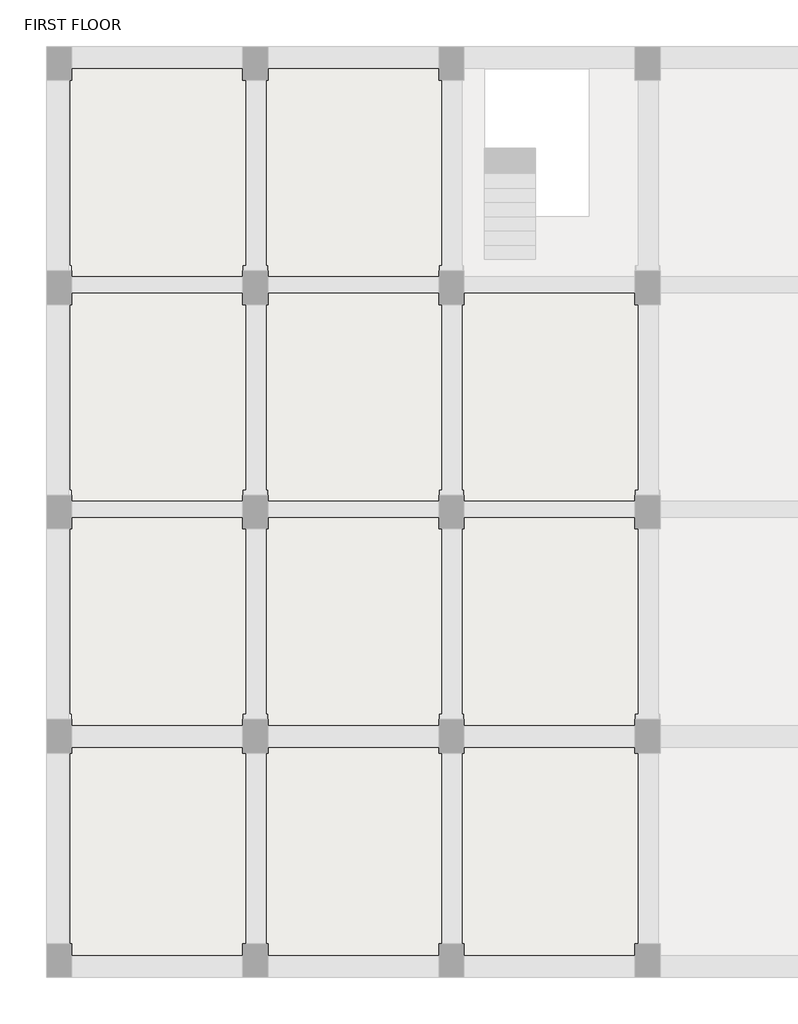
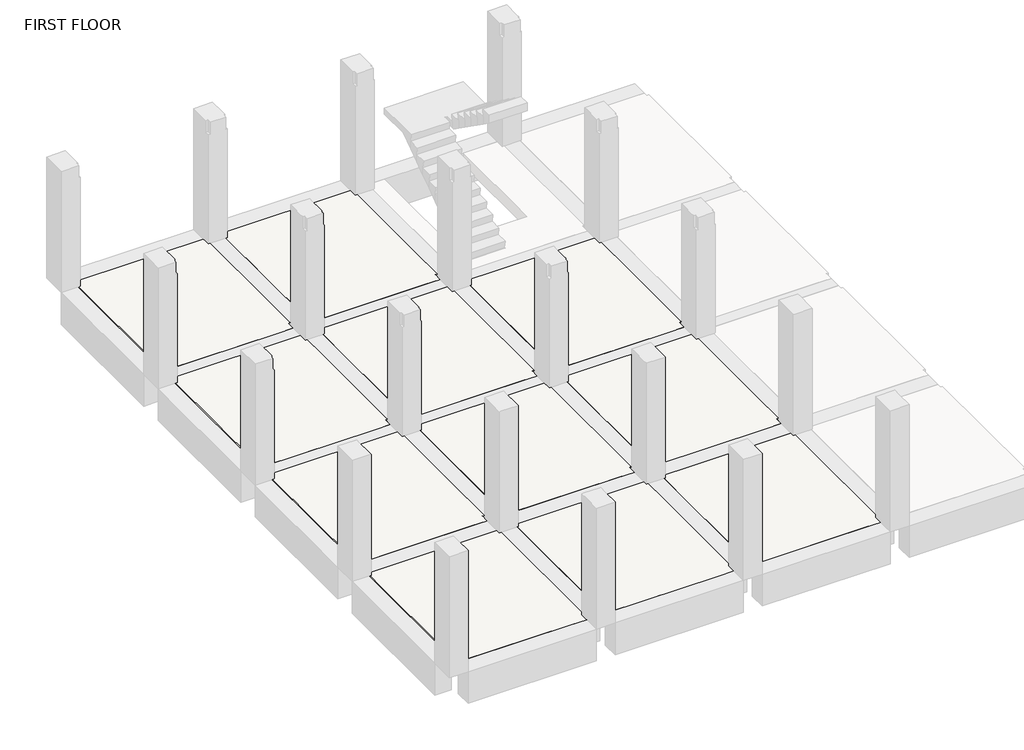
# One storey, part 1 of 4: 21 slabs.
"""IFC4 building model written with IfcOpenShell, lengths in millimetres."""

from ifc_helpers import new_model, si_unit, origin, place, context, project, spatial, faceted_brep, element, save

model = new_model("IFC4")

# Units and contexts
model_context = context("Model", 3, world=origin())
ifc_project = project(units=[si_unit("LENGTHUNIT", "METRE", prefix="MILLI")], contexts=[model_context])

# Site, building, storey
site = spatial("IfcSite", under=ifc_project)
building = spatial("IfcBuilding", under=site)
storey = spatial("IfcBuildingStorey", under=building, Name="FIRST FLOOR", Elevation=3048.0)

# Slabs
placement = place(None, origin())
element("IfcSlab", 1, ObjectType="Generic 300mm", at=placement, inside=storey, context=model_context, shape_type="Brep", body=[
    faceted_brep([(955.1115906, 11203.1212443, 2748.0), (955.1115906, 11103.1212443, 2748.0), (955.1115906, 7803.1212443, 2748.0), (930.1115906, 7803.1212443, 2748.0), (905.1115906, 7803.1212443, 2748.0), (905.1115906, 7603.1212443, 2748.0), (530.1115906, 7603.1212443, 2748.0), (-2144.8884094, 7603.1212443, 2748.0), (-2144.8884094, 7803.1212443, 2748.0), (-2169.8884094, 7803.1212443, 2748.0), (-2169.8884094, 11103.1212443, 2748.0), (-2169.8884094, 11203.1212443, 2748.0), (-2144.8884094, 11203.1212443, 2748.0), (-2144.8884094, 11303.1212443, 2748.0), (905.1115906, 11303.1212443, 2748.0), (905.1115906, 11203.1212443, 2748.0), (955.1115906, 11203.1212443, 3048.0), (905.1115906, 11203.1212443, 3048.0), (905.1115906, 11303.1212443, 3048.0), (-2144.8884094, 11303.1212443, 3048.0), (-2144.8884094, 11203.1212443, 3048.0), (-2169.8884094, 11203.1212443, 3048.0), (-2169.8884094, 11103.1212443, 3048.0), (-2169.8884094, 7803.1212443, 3048.0), (-2144.8884094, 7803.1212443, 3048.0), (-2144.8884094, 7703.1212443, 3048.0), (-2144.8884094, 7603.1212443, 3048.0), (530.1115906, 7603.1212443, 3048.0), (905.1115906, 7603.1212443, 3048.0), (905.1115906, 7703.1212443, 3048.0), (905.1115906, 7803.1212443, 3048.0), (930.1115906, 7803.1212443, 3048.0), (955.1115906, 7803.1212443, 3048.0), (955.1115906, 11103.1212443, 3048.0)], [[[0, 1, 2, 3, 4, 5, 6, 7, 8, 9, 10, 11, 12, 13, 14, 15]], [[16, 17, 18, 19, 20, 21, 22, 23, 24, 25, 26, 27, 28, 29, 30, 31, 32, 33]], [[2, 1, 0, 16, 33, 32]], [[4, 3, 2, 32, 31, 30]], [[5, 4, 30, 29, 28]], [[6, 5, 28, 27]], [[7, 6, 27, 26]], [[8, 7, 26, 25, 24]], [[9, 8, 24, 23]], [[11, 10, 9, 23, 22, 21]], [[12, 11, 21, 20]], [[13, 12, 20, 19]], [[14, 13, 19, 18]], [[15, 14, 18, 17]], [[0, 15, 17, 16]]]),
])
element("IfcSlab", 2, ObjectType="Generic 300mm", at=placement, inside=storey, context=model_context, shape_type="Brep", body=[
    faceted_brep([(-2544.8884094, 11203.1212443, 2748.0), (-2544.8884094, 11103.1212443, 2748.0), (-2544.8884094, 7803.1212443, 2748.0), (-2569.8884094, 7803.1212443, 2748.0), (-2594.8884094, 7803.1212443, 2748.0), (-2594.8884094, 7603.1212443, 2748.0), (-2969.8884094, 7603.1212443, 2748.0), (-5644.8884094, 7603.1212443, 2748.0), (-5644.8884094, 7803.1212443, 2748.0), (-5669.8884094, 7803.1212443, 2748.0), (-5669.8884094, 11103.1212443, 2748.0), (-5669.8884094, 11203.1212443, 2748.0), (-5644.8884094, 11203.1212443, 2748.0), (-5644.8884094, 11303.1212443, 2748.0), (-2594.8884094, 11303.1212443, 2748.0), (-2594.8884094, 11203.1212443, 2748.0), (-2544.8884094, 11203.1212443, 3048.0), (-2594.8884094, 11203.1212443, 3048.0), (-2594.8884094, 11303.1212443, 3048.0), (-5644.8884094, 11303.1212443, 3048.0), (-5644.8884094, 11203.1212443, 3048.0), (-5669.8884094, 11203.1212443, 3048.0), (-5669.8884094, 11103.1212443, 3048.0), (-5669.8884094, 7803.1212443, 3048.0), (-5644.8884094, 7803.1212443, 3048.0), (-5644.8884094, 7703.1212443, 3048.0), (-5644.8884094, 7603.1212443, 3048.0), (-2969.8884094, 7603.1212443, 3048.0), (-2594.8884094, 7603.1212443, 3048.0), (-2594.8884094, 7703.1212443, 3048.0), (-2594.8884094, 7803.1212443, 3048.0), (-2569.8884094, 7803.1212443, 3048.0), (-2544.8884094, 7803.1212443, 3048.0), (-2544.8884094, 11103.1212443, 3048.0)], [[[0, 1, 2, 3, 4, 5, 6, 7, 8, 9, 10, 11, 12, 13, 14, 15]], [[16, 17, 18, 19, 20, 21, 22, 23, 24, 25, 26, 27, 28, 29, 30, 31, 32, 33]], [[2, 1, 0, 16, 33, 32]], [[4, 3, 2, 32, 31, 30]], [[5, 4, 30, 29, 28]], [[6, 5, 28, 27]], [[7, 6, 27, 26]], [[8, 7, 26, 25, 24]], [[9, 8, 24, 23]], [[11, 10, 9, 23, 22, 21]], [[12, 11, 21, 20]], [[13, 12, 20, 19]], [[14, 13, 19, 18]], [[15, 14, 18, 17]], [[0, 15, 17, 16]]]),
])
element("IfcSlab", 3, ObjectType="Generic 300mm", at=placement, inside=storey, context=model_context, shape_type="Brep", body=[
    faceted_brep([(-6044.8884094, 11203.1212443, 2748.0), (-6044.8884094, 11103.1212443, 2748.0), (-6044.8884094, 7803.1212443, 2748.0), (-6069.8884094, 7803.1212443, 2748.0), (-6094.8884094, 7803.1212443, 2748.0), (-6094.8884094, 7603.1212443, 2748.0), (-6469.8884094, 7603.1212443, 2748.0), (-9144.8884094, 7603.1212443, 2748.0), (-9144.8884094, 7803.1212443, 2748.0), (-9169.8884094, 7803.1212443, 2748.0), (-9169.8884094, 11103.1212443, 2748.0), (-9169.8884094, 11203.1212443, 2748.0), (-9144.8884094, 11203.1212443, 2748.0), (-9144.8884094, 11303.1212443, 2748.0), (-6094.8884094, 11303.1212443, 2748.0), (-6094.8884094, 11203.1212443, 2748.0), (-6044.8884094, 11203.1212443, 3048.0), (-6094.8884094, 11203.1212443, 3048.0), (-6094.8884094, 11303.1212443, 3048.0), (-9144.8884094, 11303.1212443, 3048.0), (-9144.8884094, 11203.1212443, 3048.0), (-9169.8884094, 11203.1212443, 3048.0), (-9169.8884094, 11103.1212443, 3048.0), (-9169.8884094, 7803.1212443, 3048.0), (-9144.8884094, 7803.1212443, 3048.0), (-9144.8884094, 7703.1212443, 3048.0), (-9144.8884094, 7603.1212443, 3048.0), (-6469.8884094, 7603.1212443, 3048.0), (-6094.8884094, 7603.1212443, 3048.0), (-6094.8884094, 7703.1212443, 3048.0), (-6094.8884094, 7803.1212443, 3048.0), (-6069.8884094, 7803.1212443, 3048.0), (-6044.8884094, 7803.1212443, 3048.0), (-6044.8884094, 11103.1212443, 3048.0)], [[[0, 1, 2, 3, 4, 5, 6, 7, 8, 9, 10, 11, 12, 13, 14, 15]], [[16, 17, 18, 19, 20, 21, 22, 23, 24, 25, 26, 27, 28, 29, 30, 31, 32, 33]], [[2, 1, 0, 16, 33, 32]], [[4, 3, 2, 32, 31, 30]], [[5, 4, 30, 29, 28]], [[6, 5, 28, 27]], [[7, 6, 27, 26]], [[8, 7, 26, 25, 24]], [[9, 8, 24, 23]], [[11, 10, 9, 23, 22, 21]], [[12, 11, 21, 20]], [[13, 12, 20, 19]], [[14, 13, 19, 18]], [[15, 14, 18, 17]], [[0, 15, 17, 16]]]),
])
element("IfcSlab", 4, ObjectType="Generic 300mm", at=placement, inside=storey, context=model_context, shape_type="Brep", body=[
    faceted_brep([(-6044.8884094, 7103.1212443, 2748.0), (-6044.8884094, 3703.1212443, 2748.0), (-6069.8884094, 3703.1212443, 2748.0), (-6094.8884094, 3703.1212443, 2748.0), (-6094.8884094, 3503.1212443, 2748.0), (-6469.8884094, 3503.1212443, 2748.0), (-9144.8884094, 3503.1212443, 2748.0), (-9144.8884094, 3703.1212443, 2748.0), (-9169.8884094, 3703.1212443, 2748.0), (-9169.8884094, 7103.1212443, 2748.0), (-9144.8884094, 7103.1212443, 2748.0), (-9144.8884094, 7203.1212443, 2748.0), (-6094.8884094, 7203.1212443, 2748.0), (-6094.8884094, 7103.1212443, 2748.0), (-6069.8884094, 7103.1212443, 2748.0), (-6044.8884094, 7103.1212443, 3048.0), (-6094.8884094, 7103.1212443, 3048.0), (-6094.8884094, 7203.1212443, 3048.0), (-9144.8884094, 7203.1212443, 3048.0), (-9144.8884094, 7103.1212443, 3048.0), (-9169.8884094, 7103.1212443, 3048.0), (-9169.8884094, 3703.1212443, 3048.0), (-9144.8884094, 3703.1212443, 3048.0), (-9144.8884094, 3503.1212443, 3048.0), (-6469.8884094, 3503.1212443, 3048.0), (-6094.8884094, 3503.1212443, 3048.0), (-6094.8884094, 3703.1212443, 3048.0), (-6044.8884094, 3703.1212443, 3048.0)], [[[0, 1, 2, 3, 4, 5, 6, 7, 8, 9, 10, 11, 12, 13, 14]], [[15, 16, 17, 18, 19, 20, 21, 22, 23, 24, 25, 26, 27]], [[1, 0, 15, 27]], [[3, 2, 1, 27, 26]], [[4, 3, 26, 25]], [[5, 4, 25, 24]], [[6, 5, 24, 23]], [[7, 6, 23, 22]], [[8, 7, 22, 21]], [[9, 8, 21, 20]], [[10, 9, 20, 19]], [[11, 10, 19, 18]], [[12, 11, 18, 17]], [[13, 12, 17, 16]], [[0, 14, 13, 16, 15]]]),
])
element("IfcSlab", 5, ObjectType="Generic 300mm", at=placement, inside=storey, context=model_context, shape_type="Brep", body=[
    faceted_brep([(-2544.8884094, 7103.1212443, 2748.0), (-2544.8884094, 3703.1212443, 2748.0), (-2569.8884094, 3703.1212443, 2748.0), (-2594.8884094, 3703.1212443, 2748.0), (-2594.8884094, 3503.1212443, 2748.0), (-2969.8884094, 3503.1212443, 2748.0), (-5644.8884094, 3503.1212443, 2748.0), (-5644.8884094, 3703.1212443, 2748.0), (-5669.8884094, 3703.1212443, 2748.0), (-5669.8884094, 7103.1212443, 2748.0), (-5644.8884094, 7103.1212443, 2748.0), (-5644.8884094, 7203.1212443, 2748.0), (-2594.8884094, 7203.1212443, 2748.0), (-2594.8884094, 7103.1212443, 2748.0), (-2569.8884094, 7103.1212443, 2748.0), (-2544.8884094, 7103.1212443, 3048.0), (-2594.8884094, 7103.1212443, 3048.0), (-2594.8884094, 7203.1212443, 3048.0), (-5644.8884094, 7203.1212443, 3048.0), (-5644.8884094, 7103.1212443, 3048.0), (-5669.8884094, 7103.1212443, 3048.0), (-5669.8884094, 3703.1212443, 3048.0), (-5644.8884094, 3703.1212443, 3048.0), (-5644.8884094, 3503.1212443, 3048.0), (-2969.8884094, 3503.1212443, 3048.0), (-2594.8884094, 3503.1212443, 3048.0), (-2594.8884094, 3703.1212443, 3048.0), (-2544.8884094, 3703.1212443, 3048.0)], [[[0, 1, 2, 3, 4, 5, 6, 7, 8, 9, 10, 11, 12, 13, 14]], [[15, 16, 17, 18, 19, 20, 21, 22, 23, 24, 25, 26, 27]], [[1, 0, 15, 27]], [[3, 2, 1, 27, 26]], [[4, 3, 26, 25]], [[5, 4, 25, 24]], [[6, 5, 24, 23]], [[7, 6, 23, 22]], [[8, 7, 22, 21]], [[9, 8, 21, 20]], [[10, 9, 20, 19]], [[11, 10, 19, 18]], [[12, 11, 18, 17]], [[13, 12, 17, 16]], [[0, 14, 13, 16, 15]]]),
])
element("IfcSlab", 6, ObjectType="Generic 300mm", at=placement, inside=storey, context=model_context, shape_type="Brep", body=[
    faceted_brep([(955.1115906, 7103.1212443, 2748.0), (955.1115906, 3703.1212443, 2748.0), (930.1115906, 3703.1212443, 2748.0), (905.1115906, 3703.1212443, 2748.0), (905.1115906, 3503.1212443, 2748.0), (530.1115906, 3503.1212443, 2748.0), (-2144.8884094, 3503.1212443, 2748.0), (-2144.8884094, 3703.1212443, 2748.0), (-2169.8884094, 3703.1212443, 2748.0), (-2169.8884094, 7103.1212443, 2748.0), (-2144.8884094, 7103.1212443, 2748.0), (-2144.8884094, 7203.1212443, 2748.0), (905.1115906, 7203.1212443, 2748.0), (905.1115906, 7103.1212443, 2748.0), (930.1115906, 7103.1212443, 2748.0), (955.1115906, 7103.1212443, 3048.0), (905.1115906, 7103.1212443, 3048.0), (905.1115906, 7203.1212443, 3048.0), (-2144.8884094, 7203.1212443, 3048.0), (-2144.8884094, 7103.1212443, 3048.0), (-2169.8884094, 7103.1212443, 3048.0), (-2169.8884094, 3703.1212443, 3048.0), (-2144.8884094, 3703.1212443, 3048.0), (-2144.8884094, 3503.1212443, 3048.0), (530.1115906, 3503.1212443, 3048.0), (905.1115906, 3503.1212443, 3048.0), (905.1115906, 3703.1212443, 3048.0), (955.1115906, 3703.1212443, 3048.0)], [[[0, 1, 2, 3, 4, 5, 6, 7, 8, 9, 10, 11, 12, 13, 14]], [[15, 16, 17, 18, 19, 20, 21, 22, 23, 24, 25, 26, 27]], [[1, 0, 15, 27]], [[3, 2, 1, 27, 26]], [[4, 3, 26, 25]], [[5, 4, 25, 24]], [[6, 5, 24, 23]], [[7, 6, 23, 22]], [[8, 7, 22, 21]], [[9, 8, 21, 20]], [[10, 9, 20, 19]], [[11, 10, 19, 18]], [[12, 11, 18, 17]], [[13, 12, 17, 16]], [[0, 14, 13, 16, 15]]]),
])
element("IfcSlab", 7, ObjectType="Generic 300mm", at=placement, inside=storey, context=model_context, shape_type="Brep", body=[
    faceted_brep([(955.1115906, 15203.1212443, 2748.0), (955.1115906, 15103.1212443, 2748.0), (955.1115906, 11803.1212443, 2748.0), (930.1115906, 11803.1212443, 2748.0), (905.1115906, 11803.1212443, 2748.0), (905.1115906, 11603.1212443, 2748.0), (530.1115906, 11603.1212443, 2748.0), (-2144.8884094, 11603.1212443, 2748.0), (-2144.8884094, 11803.1212443, 2748.0), (-2169.8884094, 11803.1212443, 2748.0), (-2169.8884094, 15103.1212443, 2748.0), (-2169.8884094, 15203.1212443, 2748.0), (-2144.8884094, 15203.1212443, 2748.0), (-2144.8884094, 15303.1212443, 2748.0), (905.1115906, 15303.1212443, 2748.0), (905.1115906, 15203.1212443, 2748.0), (955.1115906, 15203.1212443, 3048.0), (905.1115906, 15203.1212443, 3048.0), (905.1115906, 15303.1212443, 3048.0), (-2144.8884094, 15303.1212443, 3048.0), (-2144.8884094, 15203.1212443, 3048.0), (-2169.8884094, 15203.1212443, 3048.0), (-2169.8884094, 15103.1212443, 3048.0), (-2169.8884094, 11803.1212443, 3048.0), (-2144.8884094, 11803.1212443, 3048.0), (-2144.8884094, 11703.1212443, 3048.0), (-2144.8884094, 11603.1212443, 3048.0), (530.1115906, 11603.1212443, 3048.0), (905.1115906, 11603.1212443, 3048.0), (905.1115906, 11703.1212443, 3048.0), (905.1115906, 11803.1212443, 3048.0), (930.1115906, 11803.1212443, 3048.0), (955.1115906, 11803.1212443, 3048.0), (955.1115906, 15103.1212443, 3048.0)], [[[0, 1, 2, 3, 4, 5, 6, 7, 8, 9, 10, 11, 12, 13, 14, 15]], [[16, 17, 18, 19, 20, 21, 22, 23, 24, 25, 26, 27, 28, 29, 30, 31, 32, 33]], [[2, 1, 0, 16, 33, 32]], [[4, 3, 2, 32, 31, 30]], [[5, 4, 30, 29, 28]], [[6, 5, 28, 27]], [[7, 6, 27, 26]], [[8, 7, 26, 25, 24]], [[9, 8, 24, 23]], [[11, 10, 9, 23, 22, 21]], [[12, 11, 21, 20]], [[13, 12, 20, 19]], [[14, 13, 19, 18]], [[15, 14, 18, 17]], [[0, 15, 17, 16]]]),
])
element("IfcSlab", 8, ObjectType="Generic 300mm", at=placement, inside=storey, context=model_context, shape_type="Brep", body=[
    faceted_brep([(-2544.8884094, 19203.1212443, 2748.0), (-2544.8884094, 19103.1212443, 2748.0), (-2544.8884094, 15803.1212443, 2748.0), (-2569.8884094, 15803.1212443, 2748.0), (-2594.8884094, 15803.1212443, 2748.0), (-2594.8884094, 15603.1212443, 2748.0), (-2969.8884094, 15603.1212443, 2748.0), (-5644.8884094, 15603.1212443, 2748.0), (-5644.8884094, 15803.1212443, 2748.0), (-5669.8884094, 15803.1212443, 2748.0), (-5669.8884094, 19103.1212443, 2748.0), (-5669.8884094, 19203.1212443, 2748.0), (-5644.8884094, 19203.1212443, 2748.0), (-5644.8884094, 19303.1212443, 2748.0), (-2594.8884094, 19303.1212443, 2748.0), (-2594.8884094, 19203.1212443, 2748.0), (-2544.8884094, 19203.1212443, 3048.0), (-2594.8884094, 19203.1212443, 3048.0), (-2594.8884094, 19303.1212443, 3048.0), (-5644.8884094, 19303.1212443, 3048.0), (-5644.8884094, 19203.1212443, 3048.0), (-5669.8884094, 19203.1212443, 3048.0), (-5669.8884094, 19103.1212443, 3048.0), (-5669.8884094, 15803.1212443, 3048.0), (-5644.8884094, 15803.1212443, 3048.0), (-5644.8884094, 15703.1212443, 3048.0), (-5644.8884094, 15603.1212443, 3048.0), (-2969.8884094, 15603.1212443, 3048.0), (-2594.8884094, 15603.1212443, 3048.0), (-2594.8884094, 15703.1212443, 3048.0), (-2594.8884094, 15803.1212443, 3048.0), (-2569.8884094, 15803.1212443, 3048.0), (-2544.8884094, 15803.1212443, 3048.0), (-2544.8884094, 19103.1212443, 3048.0)], [[[0, 1, 2, 3, 4, 5, 6, 7, 8, 9, 10, 11, 12, 13, 14, 15]], [[16, 17, 18, 19, 20, 21, 22, 23, 24, 25, 26, 27, 28, 29, 30, 31, 32, 33]], [[2, 1, 0, 16, 33, 32]], [[4, 3, 2, 32, 31, 30]], [[5, 4, 30, 29, 28]], [[6, 5, 28, 27]], [[7, 6, 27, 26]], [[8, 7, 26, 25, 24]], [[9, 8, 24, 23]], [[11, 10, 9, 23, 22, 21]], [[12, 11, 21, 20]], [[13, 12, 20, 19]], [[14, 13, 19, 18]], [[15, 14, 18, 17]], [[0, 15, 17, 16]]]),
])
element("IfcSlab", 9, ObjectType="Generic 300mm", at=placement, inside=storey, context=model_context, shape_type="Brep", body=[
    faceted_brep([(-6044.8884094, 19203.1212443, 2748.0), (-6044.8884094, 19103.1212443, 2748.0), (-6044.8884094, 15803.1212443, 2748.0), (-6069.8884094, 15803.1212443, 2748.0), (-6094.8884094, 15803.1212443, 2748.0), (-6094.8884094, 15603.1212443, 2748.0), (-6469.8884094, 15603.1212443, 2748.0), (-9144.8884094, 15603.1212443, 2748.0), (-9144.8884094, 15803.1212443, 2748.0), (-9169.8884094, 15803.1212443, 2748.0), (-9169.8884094, 19103.1212443, 2748.0), (-9169.8884094, 19203.1212443, 2748.0), (-9144.8884094, 19203.1212443, 2748.0), (-9144.8884094, 19303.1212443, 2748.0), (-6094.8884094, 19303.1212443, 2748.0), (-6094.8884094, 19203.1212443, 2748.0), (-6044.8884094, 19203.1212443, 3048.0), (-6094.8884094, 19203.1212443, 3048.0), (-6094.8884094, 19303.1212443, 3048.0), (-9144.8884094, 19303.1212443, 3048.0), (-9144.8884094, 19203.1212443, 3048.0), (-9169.8884094, 19203.1212443, 3048.0), (-9169.8884094, 19103.1212443, 3048.0), (-9169.8884094, 15803.1212443, 3048.0), (-9144.8884094, 15803.1212443, 3048.0), (-9144.8884094, 15703.1212443, 3048.0), (-9144.8884094, 15603.1212443, 3048.0), (-6469.8884094, 15603.1212443, 3048.0), (-6094.8884094, 15603.1212443, 3048.0), (-6094.8884094, 15703.1212443, 3048.0), (-6094.8884094, 15803.1212443, 3048.0), (-6069.8884094, 15803.1212443, 3048.0), (-6044.8884094, 15803.1212443, 3048.0), (-6044.8884094, 19103.1212443, 3048.0)], [[[0, 1, 2, 3, 4, 5, 6, 7, 8, 9, 10, 11, 12, 13, 14, 15]], [[16, 17, 18, 19, 20, 21, 22, 23, 24, 25, 26, 27, 28, 29, 30, 31, 32, 33]], [[2, 1, 0, 16, 33, 32]], [[4, 3, 2, 32, 31, 30]], [[5, 4, 30, 29, 28]], [[6, 5, 28, 27]], [[7, 6, 27, 26]], [[8, 7, 26, 25, 24]], [[9, 8, 24, 23]], [[11, 10, 9, 23, 22, 21]], [[12, 11, 21, 20]], [[13, 12, 20, 19]], [[14, 13, 19, 18]], [[15, 14, 18, 17]], [[0, 15, 17, 16]]]),
])
element("IfcSlab", 10, ObjectType="Generic 300mm", at=placement, inside=storey, context=model_context, shape_type="Brep", body=[
    faceted_brep([(-6044.8884094, 15203.1212443, 2748.0), (-6044.8884094, 15103.1212443, 2748.0), (-6044.8884094, 11803.1212443, 2748.0), (-6069.8884094, 11803.1212443, 2748.0), (-6094.8884094, 11803.1212443, 2748.0), (-6094.8884094, 11603.1212443, 2748.0), (-6469.8884094, 11603.1212443, 2748.0), (-9144.8884094, 11603.1212443, 2748.0), (-9144.8884094, 11803.1212443, 2748.0), (-9169.8884094, 11803.1212443, 2748.0), (-9169.8884094, 15103.1212443, 2748.0), (-9169.8884094, 15203.1212443, 2748.0), (-9144.8884094, 15203.1212443, 2748.0), (-9144.8884094, 15303.1212443, 2748.0), (-6094.8884094, 15303.1212443, 2748.0), (-6094.8884094, 15203.1212443, 2748.0), (-6044.8884094, 15203.1212443, 3048.0), (-6094.8884094, 15203.1212443, 3048.0), (-6094.8884094, 15303.1212443, 3048.0), (-9144.8884094, 15303.1212443, 3048.0), (-9144.8884094, 15203.1212443, 3048.0), (-9169.8884094, 15203.1212443, 3048.0), (-9169.8884094, 15103.1212443, 3048.0), (-9169.8884094, 11803.1212443, 3048.0), (-9144.8884094, 11803.1212443, 3048.0), (-9144.8884094, 11703.1212443, 3048.0), (-9144.8884094, 11603.1212443, 3048.0), (-6469.8884094, 11603.1212443, 3048.0), (-6094.8884094, 11603.1212443, 3048.0), (-6094.8884094, 11703.1212443, 3048.0), (-6094.8884094, 11803.1212443, 3048.0), (-6069.8884094, 11803.1212443, 3048.0), (-6044.8884094, 11803.1212443, 3048.0), (-6044.8884094, 15103.1212443, 3048.0)], [[[0, 1, 2, 3, 4, 5, 6, 7, 8, 9, 10, 11, 12, 13, 14, 15]], [[16, 17, 18, 19, 20, 21, 22, 23, 24, 25, 26, 27, 28, 29, 30, 31, 32, 33]], [[2, 1, 0, 16, 33, 32]], [[4, 3, 2, 32, 31, 30]], [[5, 4, 30, 29, 28]], [[6, 5, 28, 27]], [[7, 6, 27, 26]], [[8, 7, 26, 25, 24]], [[9, 8, 24, 23]], [[11, 10, 9, 23, 22, 21]], [[12, 11, 21, 20]], [[13, 12, 20, 19]], [[14, 13, 19, 18]], [[15, 14, 18, 17]], [[0, 15, 17, 16]]]),
])
element("IfcSlab", 11, ObjectType="Generic 300mm", at=placement, inside=storey, context=model_context, shape_type="Brep", body=[
    faceted_brep([(-2544.8884094, 15203.1212443, 2748.0), (-2544.8884094, 15103.1212443, 2748.0), (-2544.8884094, 11803.1212443, 2748.0), (-2569.8884094, 11803.1212443, 2748.0), (-2594.8884094, 11803.1212443, 2748.0), (-2594.8884094, 11603.1212443, 2748.0), (-2969.8884094, 11603.1212443, 2748.0), (-5644.8884094, 11603.1212443, 2748.0), (-5644.8884094, 11803.1212443, 2748.0), (-5669.8884094, 11803.1212443, 2748.0), (-5669.8884094, 15103.1212443, 2748.0), (-5669.8884094, 15203.1212443, 2748.0), (-5644.8884094, 15203.1212443, 2748.0), (-5644.8884094, 15303.1212443, 2748.0), (-2594.8884094, 15303.1212443, 2748.0), (-2594.8884094, 15203.1212443, 2748.0), (-2544.8884094, 15203.1212443, 3048.0), (-2594.8884094, 15203.1212443, 3048.0), (-2594.8884094, 15303.1212443, 3048.0), (-5644.8884094, 15303.1212443, 3048.0), (-5644.8884094, 15203.1212443, 3048.0), (-5669.8884094, 15203.1212443, 3048.0), (-5669.8884094, 15103.1212443, 3048.0), (-5669.8884094, 11803.1212443, 3048.0), (-5644.8884094, 11803.1212443, 3048.0), (-5644.8884094, 11703.1212443, 3048.0), (-5644.8884094, 11603.1212443, 3048.0), (-2969.8884094, 11603.1212443, 3048.0), (-2594.8884094, 11603.1212443, 3048.0), (-2594.8884094, 11703.1212443, 3048.0), (-2594.8884094, 11803.1212443, 3048.0), (-2569.8884094, 11803.1212443, 3048.0), (-2544.8884094, 11803.1212443, 3048.0), (-2544.8884094, 15103.1212443, 3048.0)], [[[0, 1, 2, 3, 4, 5, 6, 7, 8, 9, 10, 11, 12, 13, 14, 15]], [[16, 17, 18, 19, 20, 21, 22, 23, 24, 25, 26, 27, 28, 29, 30, 31, 32, 33]], [[2, 1, 0, 16, 33, 32]], [[4, 3, 2, 32, 31, 30]], [[5, 4, 30, 29, 28]], [[6, 5, 28, 27]], [[7, 6, 27, 26]], [[8, 7, 26, 25, 24]], [[9, 8, 24, 23]], [[11, 10, 9, 23, 22, 21]], [[12, 11, 21, 20]], [[13, 12, 20, 19]], [[14, 13, 19, 18]], [[15, 14, 18, 17]], [[0, 15, 17, 16]]]),
])
element("IfcSlab", 12, ObjectType="Generic 300mm", at=placement, inside=storey, context=model_context, shape_type="Brep", body=[
    faceted_brep([(955.1115906, 11203.1212443, 2748.0), (955.1115906, 11103.1212443, 2748.0), (955.1115906, 7803.1212443, 2748.0), (930.1115906, 7803.1212443, 2748.0), (905.1115906, 7803.1212443, 2748.0), (905.1115906, 7603.1212443, 2748.0), (530.1115906, 7603.1212443, 2748.0), (-2144.8884094, 7603.1212443, 2748.0), (-2144.8884094, 7803.1212443, 2748.0), (-2169.8884094, 7803.1212443, 2748.0), (-2169.8884094, 11103.1212443, 2748.0), (-2169.8884094, 11203.1212443, 2748.0), (-2144.8884094, 11203.1212443, 2748.0), (-2144.8884094, 11303.1212443, 2748.0), (905.1115906, 11303.1212443, 2748.0), (905.1115906, 11203.1212443, 2748.0), (955.1115906, 11203.1212443, 3048.0), (905.1115906, 11203.1212443, 3048.0), (905.1115906, 11303.1212443, 3048.0), (-2144.8884094, 11303.1212443, 3048.0), (-2144.8884094, 11203.1212443, 3048.0), (-2169.8884094, 11203.1212443, 3048.0), (-2169.8884094, 11103.1212443, 3048.0), (-2169.8884094, 7803.1212443, 3048.0), (-2144.8884094, 7803.1212443, 3048.0), (-2144.8884094, 7703.1212443, 3048.0), (-2144.8884094, 7603.1212443, 3048.0), (530.1115906, 7603.1212443, 3048.0), (905.1115906, 7603.1212443, 3048.0), (905.1115906, 7703.1212443, 3048.0), (905.1115906, 7803.1212443, 3048.0), (930.1115906, 7803.1212443, 3048.0), (955.1115906, 7803.1212443, 3048.0), (955.1115906, 11103.1212443, 3048.0)], [[[0, 1, 2, 3, 4, 5, 6, 7, 8, 9, 10, 11, 12, 13, 14, 15]], [[16, 17, 18, 19, 20, 21, 22, 23, 24, 25, 26, 27, 28, 29, 30, 31, 32, 33]], [[2, 1, 0, 16, 33, 32]], [[4, 3, 2, 32, 31, 30]], [[5, 4, 30, 29, 28]], [[6, 5, 28, 27]], [[7, 6, 27, 26]], [[8, 7, 26, 25, 24]], [[9, 8, 24, 23]], [[11, 10, 9, 23, 22, 21]], [[12, 11, 21, 20]], [[13, 12, 20, 19]], [[14, 13, 19, 18]], [[15, 14, 18, 17]], [[0, 15, 17, 16]]]),
])
element("IfcSlab", 13, ObjectType="Generic 300mm", at=placement, inside=storey, context=model_context, shape_type="Brep", body=[
    faceted_brep([(-2544.8884094, 11203.1212443, 2748.0), (-2544.8884094, 11103.1212443, 2748.0), (-2544.8884094, 7803.1212443, 2748.0), (-2569.8884094, 7803.1212443, 2748.0), (-2594.8884094, 7803.1212443, 2748.0), (-2594.8884094, 7603.1212443, 2748.0), (-2969.8884094, 7603.1212443, 2748.0), (-5644.8884094, 7603.1212443, 2748.0), (-5644.8884094, 7803.1212443, 2748.0), (-5669.8884094, 7803.1212443, 2748.0), (-5669.8884094, 11103.1212443, 2748.0), (-5669.8884094, 11203.1212443, 2748.0), (-5644.8884094, 11203.1212443, 2748.0), (-5644.8884094, 11303.1212443, 2748.0), (-2594.8884094, 11303.1212443, 2748.0), (-2594.8884094, 11203.1212443, 2748.0), (-2544.8884094, 11203.1212443, 3048.0), (-2594.8884094, 11203.1212443, 3048.0), (-2594.8884094, 11303.1212443, 3048.0), (-5644.8884094, 11303.1212443, 3048.0), (-5644.8884094, 11203.1212443, 3048.0), (-5669.8884094, 11203.1212443, 3048.0), (-5669.8884094, 11103.1212443, 3048.0), (-5669.8884094, 7803.1212443, 3048.0), (-5644.8884094, 7803.1212443, 3048.0), (-5644.8884094, 7703.1212443, 3048.0), (-5644.8884094, 7603.1212443, 3048.0), (-2969.8884094, 7603.1212443, 3048.0), (-2594.8884094, 7603.1212443, 3048.0), (-2594.8884094, 7703.1212443, 3048.0), (-2594.8884094, 7803.1212443, 3048.0), (-2569.8884094, 7803.1212443, 3048.0), (-2544.8884094, 7803.1212443, 3048.0), (-2544.8884094, 11103.1212443, 3048.0)], [[[0, 1, 2, 3, 4, 5, 6, 7, 8, 9, 10, 11, 12, 13, 14, 15]], [[16, 17, 18, 19, 20, 21, 22, 23, 24, 25, 26, 27, 28, 29, 30, 31, 32, 33]], [[2, 1, 0, 16, 33, 32]], [[4, 3, 2, 32, 31, 30]], [[5, 4, 30, 29, 28]], [[6, 5, 28, 27]], [[7, 6, 27, 26]], [[8, 7, 26, 25, 24]], [[9, 8, 24, 23]], [[11, 10, 9, 23, 22, 21]], [[12, 11, 21, 20]], [[13, 12, 20, 19]], [[14, 13, 19, 18]], [[15, 14, 18, 17]], [[0, 15, 17, 16]]]),
])
element("IfcSlab", 14, ObjectType="Generic 300mm", at=placement, inside=storey, context=model_context, shape_type="Brep", body=[
    faceted_brep([(-6044.8884094, 11203.1212443, 2748.0), (-6044.8884094, 11103.1212443, 2748.0), (-6044.8884094, 7803.1212443, 2748.0), (-6069.8884094, 7803.1212443, 2748.0), (-6094.8884094, 7803.1212443, 2748.0), (-6094.8884094, 7603.1212443, 2748.0), (-6469.8884094, 7603.1212443, 2748.0), (-9144.8884094, 7603.1212443, 2748.0), (-9144.8884094, 7803.1212443, 2748.0), (-9169.8884094, 7803.1212443, 2748.0), (-9169.8884094, 11103.1212443, 2748.0), (-9169.8884094, 11203.1212443, 2748.0), (-9144.8884094, 11203.1212443, 2748.0), (-9144.8884094, 11303.1212443, 2748.0), (-6094.8884094, 11303.1212443, 2748.0), (-6094.8884094, 11203.1212443, 2748.0), (-6044.8884094, 11203.1212443, 3048.0), (-6094.8884094, 11203.1212443, 3048.0), (-6094.8884094, 11303.1212443, 3048.0), (-9144.8884094, 11303.1212443, 3048.0), (-9144.8884094, 11203.1212443, 3048.0), (-9169.8884094, 11203.1212443, 3048.0), (-9169.8884094, 11103.1212443, 3048.0), (-9169.8884094, 7803.1212443, 3048.0), (-9144.8884094, 7803.1212443, 3048.0), (-9144.8884094, 7703.1212443, 3048.0), (-9144.8884094, 7603.1212443, 3048.0), (-6469.8884094, 7603.1212443, 3048.0), (-6094.8884094, 7603.1212443, 3048.0), (-6094.8884094, 7703.1212443, 3048.0), (-6094.8884094, 7803.1212443, 3048.0), (-6069.8884094, 7803.1212443, 3048.0), (-6044.8884094, 7803.1212443, 3048.0), (-6044.8884094, 11103.1212443, 3048.0)], [[[0, 1, 2, 3, 4, 5, 6, 7, 8, 9, 10, 11, 12, 13, 14, 15]], [[16, 17, 18, 19, 20, 21, 22, 23, 24, 25, 26, 27, 28, 29, 30, 31, 32, 33]], [[2, 1, 0, 16, 33, 32]], [[4, 3, 2, 32, 31, 30]], [[5, 4, 30, 29, 28]], [[6, 5, 28, 27]], [[7, 6, 27, 26]], [[8, 7, 26, 25, 24]], [[9, 8, 24, 23]], [[11, 10, 9, 23, 22, 21]], [[12, 11, 21, 20]], [[13, 12, 20, 19]], [[14, 13, 19, 18]], [[15, 14, 18, 17]], [[0, 15, 17, 16]]]),
])
element("IfcSlab", 15, ObjectType="Generic 300mm", at=placement, inside=storey, context=model_context, shape_type="Brep", body=[
    faceted_brep([(-6044.8884094, 7103.1212443, 2748.0), (-6044.8884094, 3703.1212443, 2748.0), (-6069.8884094, 3703.1212443, 2748.0), (-6094.8884094, 3703.1212443, 2748.0), (-6094.8884094, 3503.1212443, 2748.0), (-6469.8884094, 3503.1212443, 2748.0), (-9144.8884094, 3503.1212443, 2748.0), (-9144.8884094, 3703.1212443, 2748.0), (-9169.8884094, 3703.1212443, 2748.0), (-9169.8884094, 7103.1212443, 2748.0), (-9144.8884094, 7103.1212443, 2748.0), (-9144.8884094, 7203.1212443, 2748.0), (-6094.8884094, 7203.1212443, 2748.0), (-6094.8884094, 7103.1212443, 2748.0), (-6069.8884094, 7103.1212443, 2748.0), (-6044.8884094, 7103.1212443, 3048.0), (-6094.8884094, 7103.1212443, 3048.0), (-6094.8884094, 7203.1212443, 3048.0), (-9144.8884094, 7203.1212443, 3048.0), (-9144.8884094, 7103.1212443, 3048.0), (-9169.8884094, 7103.1212443, 3048.0), (-9169.8884094, 3703.1212443, 3048.0), (-9144.8884094, 3703.1212443, 3048.0), (-9144.8884094, 3503.1212443, 3048.0), (-6469.8884094, 3503.1212443, 3048.0), (-6094.8884094, 3503.1212443, 3048.0), (-6094.8884094, 3703.1212443, 3048.0), (-6044.8884094, 3703.1212443, 3048.0)], [[[0, 1, 2, 3, 4, 5, 6, 7, 8, 9, 10, 11, 12, 13, 14]], [[15, 16, 17, 18, 19, 20, 21, 22, 23, 24, 25, 26, 27]], [[1, 0, 15, 27]], [[3, 2, 1, 27, 26]], [[4, 3, 26, 25]], [[5, 4, 25, 24]], [[6, 5, 24, 23]], [[7, 6, 23, 22]], [[8, 7, 22, 21]], [[9, 8, 21, 20]], [[10, 9, 20, 19]], [[11, 10, 19, 18]], [[12, 11, 18, 17]], [[13, 12, 17, 16]], [[0, 14, 13, 16, 15]]]),
])
element("IfcSlab", 16, ObjectType="Generic 300mm", at=placement, inside=storey, context=model_context, shape_type="Brep", body=[
    faceted_brep([(-2544.8884094, 7103.1212443, 2748.0), (-2544.8884094, 3703.1212443, 2748.0), (-2569.8884094, 3703.1212443, 2748.0), (-2594.8884094, 3703.1212443, 2748.0), (-2594.8884094, 3503.1212443, 2748.0), (-2969.8884094, 3503.1212443, 2748.0), (-5644.8884094, 3503.1212443, 2748.0), (-5644.8884094, 3703.1212443, 2748.0), (-5669.8884094, 3703.1212443, 2748.0), (-5669.8884094, 7103.1212443, 2748.0), (-5644.8884094, 7103.1212443, 2748.0), (-5644.8884094, 7203.1212443, 2748.0), (-2594.8884094, 7203.1212443, 2748.0), (-2594.8884094, 7103.1212443, 2748.0), (-2569.8884094, 7103.1212443, 2748.0), (-2544.8884094, 7103.1212443, 3048.0), (-2594.8884094, 7103.1212443, 3048.0), (-2594.8884094, 7203.1212443, 3048.0), (-5644.8884094, 7203.1212443, 3048.0), (-5644.8884094, 7103.1212443, 3048.0), (-5669.8884094, 7103.1212443, 3048.0), (-5669.8884094, 3703.1212443, 3048.0), (-5644.8884094, 3703.1212443, 3048.0), (-5644.8884094, 3503.1212443, 3048.0), (-2969.8884094, 3503.1212443, 3048.0), (-2594.8884094, 3503.1212443, 3048.0), (-2594.8884094, 3703.1212443, 3048.0), (-2544.8884094, 3703.1212443, 3048.0)], [[[0, 1, 2, 3, 4, 5, 6, 7, 8, 9, 10, 11, 12, 13, 14]], [[15, 16, 17, 18, 19, 20, 21, 22, 23, 24, 25, 26, 27]], [[1, 0, 15, 27]], [[3, 2, 1, 27, 26]], [[4, 3, 26, 25]], [[5, 4, 25, 24]], [[6, 5, 24, 23]], [[7, 6, 23, 22]], [[8, 7, 22, 21]], [[9, 8, 21, 20]], [[10, 9, 20, 19]], [[11, 10, 19, 18]], [[12, 11, 18, 17]], [[13, 12, 17, 16]], [[0, 14, 13, 16, 15]]]),
])
element("IfcSlab", 17, ObjectType="Generic 300mm", at=placement, inside=storey, context=model_context, shape_type="Brep", body=[
    faceted_brep([(955.1115906, 7103.1212443, 2748.0), (955.1115906, 3703.1212443, 2748.0), (930.1115906, 3703.1212443, 2748.0), (905.1115906, 3703.1212443, 2748.0), (905.1115906, 3503.1212443, 2748.0), (530.1115906, 3503.1212443, 2748.0), (-2144.8884094, 3503.1212443, 2748.0), (-2144.8884094, 3703.1212443, 2748.0), (-2169.8884094, 3703.1212443, 2748.0), (-2169.8884094, 7103.1212443, 2748.0), (-2144.8884094, 7103.1212443, 2748.0), (-2144.8884094, 7203.1212443, 2748.0), (905.1115906, 7203.1212443, 2748.0), (905.1115906, 7103.1212443, 2748.0), (930.1115906, 7103.1212443, 2748.0), (955.1115906, 7103.1212443, 3048.0), (905.1115906, 7103.1212443, 3048.0), (905.1115906, 7203.1212443, 3048.0), (-2144.8884094, 7203.1212443, 3048.0), (-2144.8884094, 7103.1212443, 3048.0), (-2169.8884094, 7103.1212443, 3048.0), (-2169.8884094, 3703.1212443, 3048.0), (-2144.8884094, 3703.1212443, 3048.0), (-2144.8884094, 3503.1212443, 3048.0), (530.1115906, 3503.1212443, 3048.0), (905.1115906, 3503.1212443, 3048.0), (905.1115906, 3703.1212443, 3048.0), (955.1115906, 3703.1212443, 3048.0)], [[[0, 1, 2, 3, 4, 5, 6, 7, 8, 9, 10, 11, 12, 13, 14]], [[15, 16, 17, 18, 19, 20, 21, 22, 23, 24, 25, 26, 27]], [[1, 0, 15, 27]], [[3, 2, 1, 27, 26]], [[4, 3, 26, 25]], [[5, 4, 25, 24]], [[6, 5, 24, 23]], [[7, 6, 23, 22]], [[8, 7, 22, 21]], [[9, 8, 21, 20]], [[10, 9, 20, 19]], [[11, 10, 19, 18]], [[12, 11, 18, 17]], [[13, 12, 17, 16]], [[0, 14, 13, 16, 15]]]),
])
element("IfcSlab", 18, ObjectType="Generic 300mm", at=placement, inside=storey, context=model_context, shape_type="Brep", body=[
    faceted_brep([(955.1115906, 15203.1212443, 2748.0), (955.1115906, 15103.1212443, 2748.0), (955.1115906, 11803.1212443, 2748.0), (930.1115906, 11803.1212443, 2748.0), (905.1115906, 11803.1212443, 2748.0), (905.1115906, 11603.1212443, 2748.0), (530.1115906, 11603.1212443, 2748.0), (-2144.8884094, 11603.1212443, 2748.0), (-2144.8884094, 11803.1212443, 2748.0), (-2169.8884094, 11803.1212443, 2748.0), (-2169.8884094, 15103.1212443, 2748.0), (-2169.8884094, 15203.1212443, 2748.0), (-2144.8884094, 15203.1212443, 2748.0), (-2144.8884094, 15303.1212443, 2748.0), (905.1115906, 15303.1212443, 2748.0), (905.1115906, 15203.1212443, 2748.0), (955.1115906, 15203.1212443, 3048.0), (905.1115906, 15203.1212443, 3048.0), (905.1115906, 15303.1212443, 3048.0), (-2144.8884094, 15303.1212443, 3048.0), (-2144.8884094, 15203.1212443, 3048.0), (-2169.8884094, 15203.1212443, 3048.0), (-2169.8884094, 15103.1212443, 3048.0), (-2169.8884094, 11803.1212443, 3048.0), (-2144.8884094, 11803.1212443, 3048.0), (-2144.8884094, 11703.1212443, 3048.0), (-2144.8884094, 11603.1212443, 3048.0), (530.1115906, 11603.1212443, 3048.0), (905.1115906, 11603.1212443, 3048.0), (905.1115906, 11703.1212443, 3048.0), (905.1115906, 11803.1212443, 3048.0), (930.1115906, 11803.1212443, 3048.0), (955.1115906, 11803.1212443, 3048.0), (955.1115906, 15103.1212443, 3048.0)], [[[0, 1, 2, 3, 4, 5, 6, 7, 8, 9, 10, 11, 12, 13, 14, 15]], [[16, 17, 18, 19, 20, 21, 22, 23, 24, 25, 26, 27, 28, 29, 30, 31, 32, 33]], [[2, 1, 0, 16, 33, 32]], [[4, 3, 2, 32, 31, 30]], [[5, 4, 30, 29, 28]], [[6, 5, 28, 27]], [[7, 6, 27, 26]], [[8, 7, 26, 25, 24]], [[9, 8, 24, 23]], [[11, 10, 9, 23, 22, 21]], [[12, 11, 21, 20]], [[13, 12, 20, 19]], [[14, 13, 19, 18]], [[15, 14, 18, 17]], [[0, 15, 17, 16]]]),
])
element("IfcSlab", 19, ObjectType="Generic 300mm", at=placement, inside=storey, context=model_context, shape_type="Brep", body=[
    faceted_brep([(-6044.8884094, 19203.1212443, 2748.0), (-6044.8884094, 19103.1212443, 2748.0), (-6044.8884094, 15803.1212443, 2748.0), (-6069.8884094, 15803.1212443, 2748.0), (-6094.8884094, 15803.1212443, 2748.0), (-6094.8884094, 15603.1212443, 2748.0), (-6469.8884094, 15603.1212443, 2748.0), (-9144.8884094, 15603.1212443, 2748.0), (-9144.8884094, 15803.1212443, 2748.0), (-9169.8884094, 15803.1212443, 2748.0), (-9169.8884094, 19103.1212443, 2748.0), (-9169.8884094, 19203.1212443, 2748.0), (-9144.8884094, 19203.1212443, 2748.0), (-9144.8884094, 19303.1212443, 2748.0), (-6094.8884094, 19303.1212443, 2748.0), (-6094.8884094, 19203.1212443, 2748.0), (-6044.8884094, 19203.1212443, 3048.0), (-6094.8884094, 19203.1212443, 3048.0), (-6094.8884094, 19303.1212443, 3048.0), (-9144.8884094, 19303.1212443, 3048.0), (-9144.8884094, 19203.1212443, 3048.0), (-9169.8884094, 19203.1212443, 3048.0), (-9169.8884094, 19103.1212443, 3048.0), (-9169.8884094, 15803.1212443, 3048.0), (-9144.8884094, 15803.1212443, 3048.0), (-9144.8884094, 15703.1212443, 3048.0), (-9144.8884094, 15603.1212443, 3048.0), (-6469.8884094, 15603.1212443, 3048.0), (-6094.8884094, 15603.1212443, 3048.0), (-6094.8884094, 15703.1212443, 3048.0), (-6094.8884094, 15803.1212443, 3048.0), (-6069.8884094, 15803.1212443, 3048.0), (-6044.8884094, 15803.1212443, 3048.0), (-6044.8884094, 19103.1212443, 3048.0)], [[[0, 1, 2, 3, 4, 5, 6, 7, 8, 9, 10, 11, 12, 13, 14, 15]], [[16, 17, 18, 19, 20, 21, 22, 23, 24, 25, 26, 27, 28, 29, 30, 31, 32, 33]], [[2, 1, 0, 16, 33, 32]], [[4, 3, 2, 32, 31, 30]], [[5, 4, 30, 29, 28]], [[6, 5, 28, 27]], [[7, 6, 27, 26]], [[8, 7, 26, 25, 24]], [[9, 8, 24, 23]], [[11, 10, 9, 23, 22, 21]], [[12, 11, 21, 20]], [[13, 12, 20, 19]], [[14, 13, 19, 18]], [[15, 14, 18, 17]], [[0, 15, 17, 16]]]),
])
element("IfcSlab", 20, ObjectType="Generic 300mm", at=placement, inside=storey, context=model_context, shape_type="Brep", body=[
    faceted_brep([(-6044.8884094, 15203.1212443, 2748.0), (-6044.8884094, 15103.1212443, 2748.0), (-6044.8884094, 11803.1212443, 2748.0), (-6069.8884094, 11803.1212443, 2748.0), (-6094.8884094, 11803.1212443, 2748.0), (-6094.8884094, 11603.1212443, 2748.0), (-6469.8884094, 11603.1212443, 2748.0), (-9144.8884094, 11603.1212443, 2748.0), (-9144.8884094, 11803.1212443, 2748.0), (-9169.8884094, 11803.1212443, 2748.0), (-9169.8884094, 15103.1212443, 2748.0), (-9169.8884094, 15203.1212443, 2748.0), (-9144.8884094, 15203.1212443, 2748.0), (-9144.8884094, 15303.1212443, 2748.0), (-6094.8884094, 15303.1212443, 2748.0), (-6094.8884094, 15203.1212443, 2748.0), (-6044.8884094, 15203.1212443, 3048.0), (-6094.8884094, 15203.1212443, 3048.0), (-6094.8884094, 15303.1212443, 3048.0), (-9144.8884094, 15303.1212443, 3048.0), (-9144.8884094, 15203.1212443, 3048.0), (-9169.8884094, 15203.1212443, 3048.0), (-9169.8884094, 15103.1212443, 3048.0), (-9169.8884094, 11803.1212443, 3048.0), (-9144.8884094, 11803.1212443, 3048.0), (-9144.8884094, 11703.1212443, 3048.0), (-9144.8884094, 11603.1212443, 3048.0), (-6469.8884094, 11603.1212443, 3048.0), (-6094.8884094, 11603.1212443, 3048.0), (-6094.8884094, 11703.1212443, 3048.0), (-6094.8884094, 11803.1212443, 3048.0), (-6069.8884094, 11803.1212443, 3048.0), (-6044.8884094, 11803.1212443, 3048.0), (-6044.8884094, 15103.1212443, 3048.0)], [[[0, 1, 2, 3, 4, 5, 6, 7, 8, 9, 10, 11, 12, 13, 14, 15]], [[16, 17, 18, 19, 20, 21, 22, 23, 24, 25, 26, 27, 28, 29, 30, 31, 32, 33]], [[2, 1, 0, 16, 33, 32]], [[4, 3, 2, 32, 31, 30]], [[5, 4, 30, 29, 28]], [[6, 5, 28, 27]], [[7, 6, 27, 26]], [[8, 7, 26, 25, 24]], [[9, 8, 24, 23]], [[11, 10, 9, 23, 22, 21]], [[12, 11, 21, 20]], [[13, 12, 20, 19]], [[14, 13, 19, 18]], [[15, 14, 18, 17]], [[0, 15, 17, 16]]]),
])
element("IfcSlab", 21, ObjectType="Generic 300mm", at=placement, inside=storey, context=model_context, shape_type="Brep", body=[
    faceted_brep([(-2544.8884094, 15203.1212443, 2748.0), (-2544.8884094, 15103.1212443, 2748.0), (-2544.8884094, 11803.1212443, 2748.0), (-2569.8884094, 11803.1212443, 2748.0), (-2594.8884094, 11803.1212443, 2748.0), (-2594.8884094, 11603.1212443, 2748.0), (-2969.8884094, 11603.1212443, 2748.0), (-5644.8884094, 11603.1212443, 2748.0), (-5644.8884094, 11803.1212443, 2748.0), (-5669.8884094, 11803.1212443, 2748.0), (-5669.8884094, 15103.1212443, 2748.0), (-5669.8884094, 15203.1212443, 2748.0), (-5644.8884094, 15203.1212443, 2748.0), (-5644.8884094, 15303.1212443, 2748.0), (-2594.8884094, 15303.1212443, 2748.0), (-2594.8884094, 15203.1212443, 2748.0), (-2544.8884094, 15203.1212443, 3048.0), (-2594.8884094, 15203.1212443, 3048.0), (-2594.8884094, 15303.1212443, 3048.0), (-5644.8884094, 15303.1212443, 3048.0), (-5644.8884094, 15203.1212443, 3048.0), (-5669.8884094, 15203.1212443, 3048.0), (-5669.8884094, 15103.1212443, 3048.0), (-5669.8884094, 11803.1212443, 3048.0), (-5644.8884094, 11803.1212443, 3048.0), (-5644.8884094, 11703.1212443, 3048.0), (-5644.8884094, 11603.1212443, 3048.0), (-2969.8884094, 11603.1212443, 3048.0), (-2594.8884094, 11603.1212443, 3048.0), (-2594.8884094, 11703.1212443, 3048.0), (-2594.8884094, 11803.1212443, 3048.0), (-2569.8884094, 11803.1212443, 3048.0), (-2544.8884094, 11803.1212443, 3048.0), (-2544.8884094, 15103.1212443, 3048.0)], [[[0, 1, 2, 3, 4, 5, 6, 7, 8, 9, 10, 11, 12, 13, 14, 15]], [[16, 17, 18, 19, 20, 21, 22, 23, 24, 25, 26, 27, 28, 29, 30, 31, 32, 33]], [[2, 1, 0, 16, 33, 32]], [[4, 3, 2, 32, 31, 30]], [[5, 4, 30, 29, 28]], [[6, 5, 28, 27]], [[7, 6, 27, 26]], [[8, 7, 26, 25, 24]], [[9, 8, 24, 23]], [[11, 10, 9, 23, 22, 21]], [[12, 11, 21, 20]], [[13, 12, 20, 19]], [[14, 13, 19, 18]], [[15, 14, 18, 17]], [[0, 15, 17, 16]]]),
])

save(model, "model.ifc")

# Revit data of these elements
# Type "Generic 300mm"
#   Function = 0
#   Layers, outside or top first: 0' - 11.81102" no material (function 1)
# Elements 1, 2, 3, 4, 5, 6, 7, 8, 9, 10, 11, 12, 13, 14, 15, 16, 17, 18, 19, 20, 21 (IfcSlab, "Generic 300mm")
#   built-in parameter 1001955 = 1.5708 (stored number, unit not read)
#   Height Offset From Level = 0' - 0"
#   built-in parameter 1001954 = 1
#   Phase Created = New Construction
#   Materials on its faces: "Default Floor"
# Materials
#   "Default Floor": colour RGB 127 127 127, transparency 0, Cost = 0
